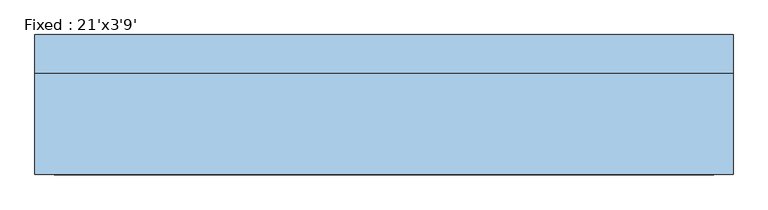
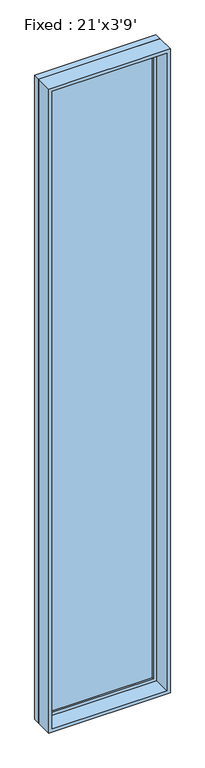
"""IFC4 building model written with IfcOpenShell, lengths in millimetres: window geometry, Fixed : 21'x3'9'."""

from ifc_helpers import new_model, si_unit, frame, origin, place, context, project, spatial, polyline, outline, extrude, source, transform, mapped, element, save


def fixed_21_x3_9_7c61b802(model_context):
    return source(origin(), model_context, "Body", "SweptSolid", [
        extrude(outline(polyline([(469.9, 66.675), (-546.1, 66.675), (-546.1, 79.375), (469.9, 79.375), (469.9, 66.675)])), frame((0.0, 0.0, 1206.5), z_axis=(0.0, 0.0, 1.0), x_axis=(1.0, 0.0, 0.0)), (0.0, 0.0, 1.0), 6273.8),
        extrude(outline(polyline([(7524.75, -590.55), (1162.05, -590.55), (1162.05, 514.35), (7524.75, 514.35), (7524.75, -590.55)]), holes=[polyline([(7480.3, -546.1), (7480.3, 469.9), (1206.5, 469.9), (1206.5, -546.1), (7480.3, -546.1)])]), frame((0.0, 50.8, 0.0), z_axis=(0.0, 1.0, 0.0), x_axis=(0.0, 0.0, 1.0)), (0.0, 0.0, 1.0), 44.45),
        extrude(outline(polyline([(7543.8, -609.6), (1143.0, -609.6), (1143.0, 533.4), (7543.8, 533.4), (7543.8, -609.6)]), holes=[polyline([(7512.05, -577.85), (7512.05, 501.65), (1174.75, 501.65), (1174.75, -577.85), (7512.05, -577.85)])]), frame((0.0, -114.3, 0.0), z_axis=(0.0, 1.0, 0.0), x_axis=(0.0, 0.0, 1.0)), (0.0, 0.0, 1.0), 165.1),
        extrude(outline(polyline([(7543.8, 533.4), (7543.8, -609.6), (1143.0, -609.6), (1143.0, 533.4), (7543.8, 533.4)]), holes=[polyline([(7524.75, 514.35), (1162.05, 514.35), (1162.05, -590.55), (7524.75, -590.55), (7524.75, 514.35)])]), frame((0.0, 50.8, 0.0), z_axis=(0.0, 1.0, 0.0), x_axis=(0.0, 0.0, 1.0)), (0.0, 0.0, 1.0), 63.5),
    ])


if __name__ == "__main__":
    model = new_model("IFC4")
    model_context = context("Model", 3, world=origin())
    ifc_project = project(units=[si_unit("LENGTHUNIT", "METRE", prefix="MILLI")], contexts=[model_context])
    site = spatial("IfcSite", under=ifc_project)
    building = spatial("IfcBuilding", under=site)
    placement = place(None, origin())
    fixed_21_x3_9_shape = fixed_21_x3_9_7c61b802(model_context)
    element("IfcWindow", 1, ObjectType="Fixed : 21'x3'9'", at=placement, inside=building, context=model_context, shape_type="MappedRepresentation", body=[
        mapped(fixed_21_x3_9_shape, transform((0.0, 0.0, 0.0), x_axis=(1.0, 0.0, 0.0), y_axis=(0.0, 1.0, 0.0), z_axis=(0.0, 0.0, 1.0))),
    ])
    save(model, "model.ifc")

# Revit data of these elements
# Type "Fixed : 21'x3'9'"
#   Type Mark = "21"
#   Construction Type Id = "GSP4R"
#   Assembly Code = "B2020100"
#   Analytic Construction = "1/8 in Pilkington single glazing"
#   Visual Light Transmittance = 0.9
#   Solar Heat Gain Coefficient = 0.78
#   Heat Transfer Coefficient (U) = 0.6496 BTU/(h·ft²·°F)
#   Height = 21' - 0"
#   Default Sill Height = 3' - 9"
#   Width = 3' - 9"
#   Window Inset = 0' - 0 3/4"
#   Define Thermal Properties by = 1
#   Glass Pane Material = Glass
#   Sash Material = Sash
#   Wall Closure = (empty or 0)
# Element 1 (IfcWindow, "Fixed : 21'x3'9'")
#   Materials on its faces: "Sash", "Glass"
# Materials
#   "Glass": class "Glass", colour RGB 0 128 192, transparency 0.75, Description = "Soda Lime Glass", Cost = 0
#   "Sash": class "Wood", colour RGB 224 178 126, transparency 0, Cost = 0
